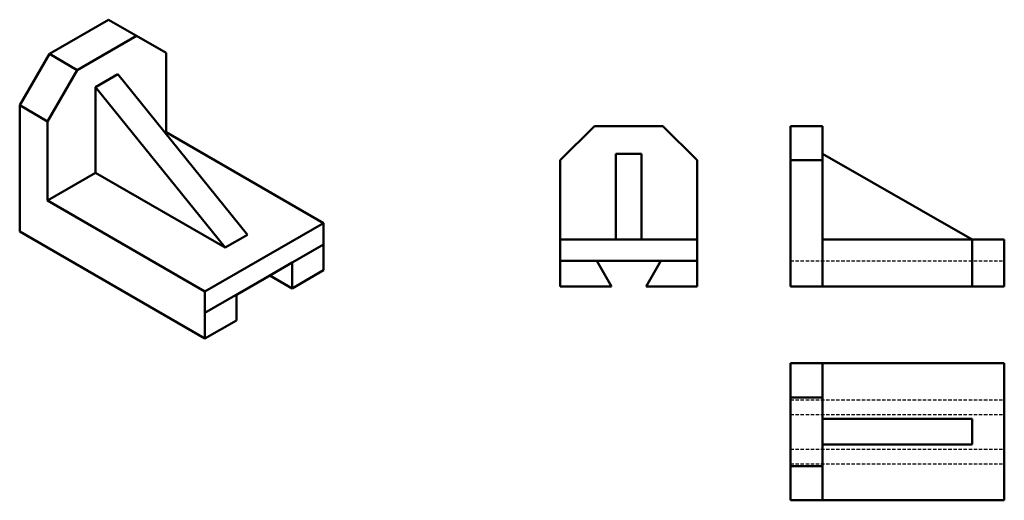
# Model space of a CAD drawing. Units: millimetres. Extents: x 4072 to 4532, y 2199 to 2424.
import ezdxf

# ---------------------------------------------------------------- set-up
doc = ezdxf.new("R2010")
doc.units = ezdxf.units.MM
doc.header["$MEASUREMENT"] = 0
doc.linetypes.add('HIDDEN', pattern=[9.525, 6.35, -3.175])
doc.layers.add('M-HIDN', color=3, linetype='HIDDEN', lineweight=25)
doc.layers.add('M-OUTL', color=7, linetype='Continuous', lineweight=50)

msp = doc.modelspace()

# ---------------------------------------------------------------- linework, layer by layer
at = {"layer": 'M-HIDN', "ltscale": 0.25}
for p, q in [((4432.34, 2311.3), (4532.34, 2311.3)), ((4432.34, 2246.45), (4532.34, 2246.45)), ((4432.34, 2239.52), (4532.34, 2239.52)), ((4432.34, 2223.38), (4532.34, 2223.38)), ((4432.34, 2216.45), (4532.34, 2216.45))]:
    msp.add_line(p, q, dxfattribs=at)
at = {"layer": 'M-OUTL'}
for p, q in [((4085.9, 2407.97), (4113.61, 2423.97)), ((4085.9, 2407.97), (4113.61, 2423.97)), ((4113.61, 2423.97), (4126.6, 2416.47)), ((4098.89, 2400.47), (4126.6, 2416.47)), ((4126.6, 2416.47), (4140.46, 2408.47)), ((4072.04, 2383.97), (4085.9, 2407.97)), ((4085.9, 2407.97), (4098.89, 2400.47)), ((4140.46, 2371.47), (4140.46, 2408.47)), ((4085.03, 2376.47), (4098.89, 2400.47)), ((4107.55, 2392.47), (4117.94, 2398.47)), ((4178.56, 2323.47), (4117.94, 2398.47)), ((4107.55, 2352.47), (4107.55, 2392.47)), ((4107.55, 2392.47), (4168.17, 2317.47)), ((4072.04, 2324.97), (4072.04, 2383.97)), ((4072.04, 2383.97), (4085.03, 2376.47)), ((4085.03, 2376.47), (4085.03, 2339.47)), ((4139.99, 2371.2), (4140.46, 2371.47)), ((4214.07, 2328.97), (4140.46, 2371.47)), ((4324.78, 2358.3), (4340.78, 2374.3)), ((4372.78, 2374.3), (4340.78, 2374.3)), ((4388.78, 2358.3), (4372.78, 2374.3)), ((4432.34, 2374.3), (4447.34, 2374.3)), ((4432.34, 2374.3), (4432.34, 2299.3)), ((4432.34, 2374.3), (4447.34, 2374.3)), ((4447.34, 2374.3), (4447.34, 2321.3)), ((4324.78, 2358.3), (4324.78, 2299.3)), ((4350.78, 2321.3), (4350.78, 2361.3)), ((4350.78, 2361.3), (4362.78, 2361.3)), ((4362.78, 2361.3), (4362.78, 2321.3)), ((4388.78, 2299.3), (4388.78, 2358.3)), ((4432.34, 2358.3), (4447.34, 2358.3)), ((4447.34, 2361.3), (4517.34, 2321.3)), ((4085.03, 2339.47), (4107.55, 2352.47)), ((4107.55, 2352.47), (4168.17, 2317.47)), ((4158.65, 2296.97), (4085.03, 2339.47)), ((4072.04, 2324.97), (4158.65, 2274.97)), ((4158.65, 2296.97), (4214.07, 2328.97)), ((4214.07, 2306.97), (4214.07, 2328.97)), ((4168.17, 2317.47), (4178.56, 2323.47)), ((4324.78, 2299.3), (4324.78, 2321.3)), ((4324.78, 2321.3), (4388.78, 2321.3)), ((4356.78, 2321.3), (4350.78, 2321.3)), ((4362.78, 2321.3), (4350.78, 2321.3)), ((4447.34, 2321.3), (4532.34, 2321.3)), ((4447.34, 2321.3), (4532.34, 2321.3)), ((4447.34, 2321.3), (4517.34, 2321.3)), ((4447.34, 2321.3), (4447.34, 2299.3)), ((4517.34, 2321.3), (4517.34, 2299.3)), ((4532.34, 2299.3), (4532.34, 2321.3)), ((4158.65, 2286.97), (4214.07, 2318.97)), ((4324.78, 2299.3), (4324.78, 2311.3)), ((4324.78, 2311.3), (4388.78, 2311.3)), ((4356.78, 2311.3), (4341.78, 2311.3)), ((4348.71, 2299.3), (4341.78, 2311.3)), ((4356.78, 2311.3), (4371.78, 2311.3)), ((4364.85, 2299.3), (4371.78, 2311.3)), ((4186.36, 2302.97), (4199.35, 2310.47)), ((4199.35, 2310.47), (4199.35, 2298.47)), ((4199.35, 2298.47), (4214.07, 2306.97)), ((4186.36, 2302.97), (4173.37, 2295.47)), ((4199.35, 2298.47), (4188.96, 2304.47)), ((4158.65, 2274.97), (4158.65, 2296.97)), ((4324.78, 2299.3), (4348.71, 2299.3)), ((4364.85, 2299.3), (4388.78, 2299.3)), ((4432.34, 2299.3), (4532.34, 2299.3)), ((4432.34, 2299.3), (4532.34, 2299.3)), ((4173.37, 2295.47), (4173.37, 2283.47)), ((4158.65, 2274.97), (4158.65, 2286.97)), ((4158.65, 2274.97), (4173.37, 2283.47)), ((4432.34, 2263.45), (4432.34, 2199.45)), ((4432.34, 2263.45), (4532.34, 2263.45)), ((4432.34, 2199.45), (4432.34, 2263.45)), ((4432.34, 2263.45), (4432.34, 2247.45)), ((4432.34, 2239.52), (4432.34, 2263.45)), ((4447.34, 2263.45), (4447.34, 2199.45)), ((4447.34, 2263.45), (4447.34, 2199.45)), ((4532.34, 2263.45), (4532.34, 2199.45)), ((4532.34, 2263.45), (4532.34, 2199.45)), ((4432.34, 2247.45), (4447.34, 2247.45)), ((4447.34, 2231.45), (4447.34, 2237.45)), ((4447.34, 2237.45), (4517.34, 2237.45)), ((4447.34, 2225.45), (4447.34, 2237.45)), ((4447.34, 2237.45), (4517.34, 2237.45)), ((4517.34, 2237.45), (4517.34, 2225.45)), ((4432.34, 2199.45), (4432.34, 2223.38)), ((4517.34, 2225.45), (4447.34, 2225.45)), ((4432.34, 2199.45), (4432.34, 2215.45)), ((4432.34, 2215.45), (4447.34, 2215.45)), ((4532.34, 2199.45), (4432.34, 2199.45))]:
    msp.add_line(p, q, dxfattribs=at)

doc.saveas('drawing.dxf')
